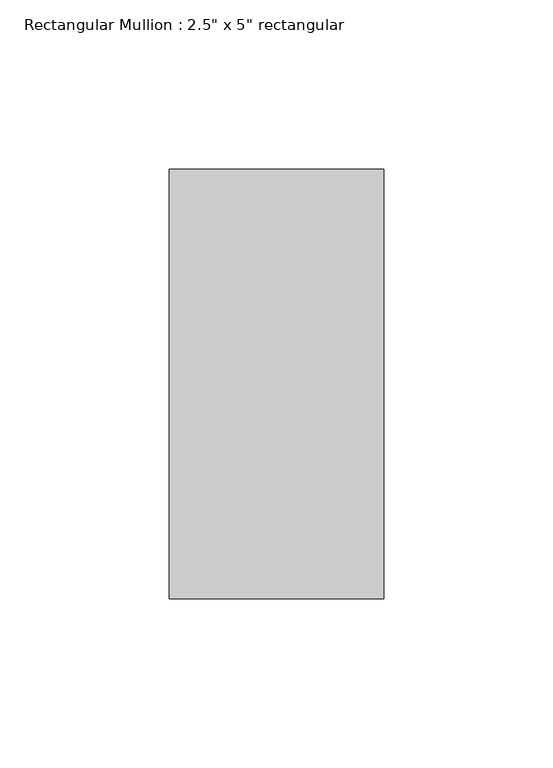
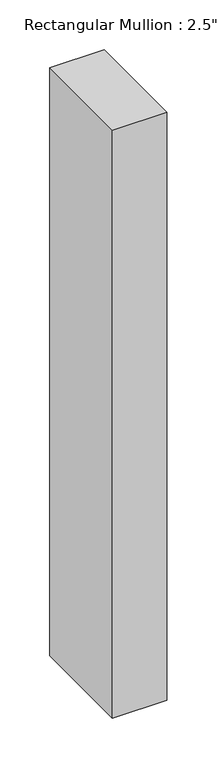
"""IFC4 building model written with IfcOpenShell, lengths in millimetres: member geometry."""

from ifc_helpers import new_model, si_unit, frame, origin, place, context, project, spatial, polyline, outline, extrude, source, transform, mapped, element, save


def member_2af9f6c8(model_context):
    return source(origin(), model_context, "Body", "SweptSolid", [
        extrude(outline(polyline([(31.75, 63.5), (31.75, -63.5), (-31.75, -63.5), (-31.75, 63.5), (31.75, 63.5)])), frame((0.0, 0.0, -724.7301773), z_axis=(0.0, 0.0, 1.0), x_axis=(1.0, 0.0, 0.0)), (0.0, 0.0, 1.0), 724.7301773),
    ])


if __name__ == "__main__":
    model = new_model("IFC4")
    model_context = context("Model", 3, world=origin())
    ifc_project = project(units=[si_unit("LENGTHUNIT", "METRE", prefix="MILLI")], contexts=[model_context])
    site = spatial("IfcSite", under=ifc_project)
    building = spatial("IfcBuilding", under=site)
    placement = place(None, origin())
    member_shape = member_2af9f6c8(model_context)
    element("IfcMember", 1, ObjectType="Rectangular Mullion : 2.5\" x 5\" rectangular", at=placement, inside=building, context=model_context, shape_type="MappedRepresentation", body=[
        mapped(member_shape, transform((0.0, 0.0, 0.0), x_axis=(1.0, 0.0, 0.0), y_axis=(0.0, 1.0, 0.0), z_axis=(0.0, 0.0, 1.0))),
    ])
    save(model, "model.ifc")

# Revit data of these elements
# Type "Rectangular Mullion : 2.5\" x 5\" rectangular"
#   built-in parameter 1007304 = 0.416667 (stored number, unit not read)
#   built-in parameter 1007301 = 0.104167 (stored number, unit not read)
#   built-in parameter 1007300 = 0.104167 (stored number, unit not read)
# Element 1 (IfcMember, "Rectangular Mullion : 2.5\" x 5\" rectangular")
#   Materials on its faces: "Aluminum"
# Materials
#   "Aluminum": class "Metal", colour RGB 247 247 247, transparency 0, Description = "Aluminum 6061", Cost = 0
